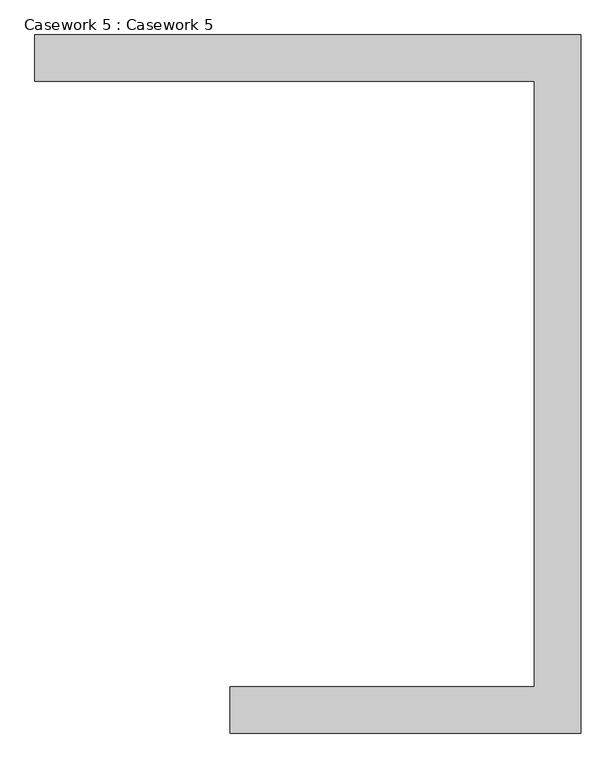
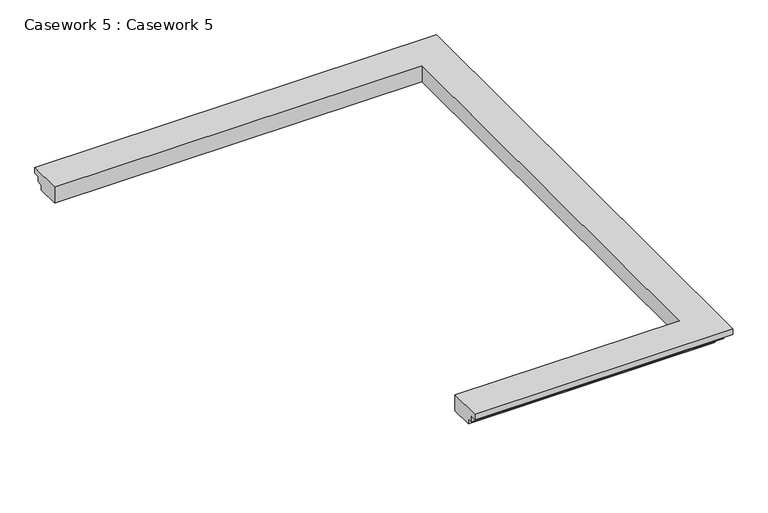
"""IFC4 building model written with IfcOpenShell, lengths in millimetres: furniture geometry, Casework 5 : Casework 5."""

from ifc_helpers import new_model, si_unit, origin, place, context, project, spatial, faceted_brep, source, transform, mapped, element, save


def casework_5_casework_5_052b1e20(model_context):
    return source(origin(), model_context, "Body", "Brep", [
        faceted_brep([(7590.7046034, -5534.1929163, 4350.0), (7590.7046034, -5934.1929163, 4350.0), (7590.7046034, -5934.1929163, 4450.0), (7590.7046034, -6034.1929163, 4450.0), (7590.7046034, -6034.1929163, 4550.0), (7590.7046034, -6134.1929163, 4550.0), (7590.7046034, -6134.1929163, 4650.0), (7590.7046034, -5534.1929163, 4650.0), (11550.7046034, -5534.1929163, 4350.0), (11550.7046034, 2340.8070837, 4350.0), (5050.7046034, 2340.8070837, 4350.0), (5050.7046034, 2740.8070837, 4350.0), (11950.7046034, 2740.8070837, 4350.0), (11950.7046034, -5934.1929163, 4350.0), (11950.7046034, -5934.1929163, 4450.0), (11950.7046034, 2740.8070837, 4450.0), (5050.7046034, 2740.8070837, 4450.0), (5050.7046034, 2840.8070837, 4450.0), (12050.7046034, 2840.8070837, 4450.0), (12050.7046034, -6034.1929163, 4450.0), (12050.7046034, -6034.1929163, 4550.0), (12050.7046034, 2840.8070837, 4550.0), (5050.7046034, 2840.8070837, 4550.0), (5050.7046034, 2940.8070837, 4550.0), (12150.7046034, 2940.8070837, 4550.0), (12150.7046034, -6134.1929163, 4550.0), (12150.7046034, -6134.1929163, 4650.0), (12150.7046034, 2940.8070837, 4650.0), (5050.7046034, 2940.8070837, 4650.0), (5050.7046034, 2340.8070837, 4650.0), (11550.7046034, 2340.8070837, 4650.0), (11550.7046034, -5534.1929163, 4650.0)], [[[0, 1, 2, 3, 4, 5, 6, 7]], [[1, 0, 8, 9, 10, 11, 12, 13]], [[2, 1, 13, 14]], [[3, 2, 14, 15, 16, 17, 18, 19]], [[4, 3, 19, 20]], [[5, 4, 20, 21, 22, 23, 24, 25]], [[6, 5, 25, 26]], [[7, 6, 26, 27, 28, 29, 30, 31]], [[0, 7, 31, 8]], [[14, 13, 12, 15]], [[20, 19, 18, 21]], [[26, 25, 24, 27]], [[8, 31, 30, 9]], [[10, 29, 28, 23, 22, 17, 16, 11]], [[15, 12, 11, 16]], [[21, 18, 17, 22]], [[27, 24, 23, 28]], [[9, 30, 29, 10]]]),
    ])


if __name__ == "__main__":
    model = new_model("IFC4")
    model_context = context("Model", 3, world=origin())
    ifc_project = project(units=[si_unit("LENGTHUNIT", "METRE", prefix="MILLI")], contexts=[model_context])
    site = spatial("IfcSite", under=ifc_project)
    building = spatial("IfcBuilding", under=site)
    placement = place(None, origin())
    casework_5_casework_5_shape = casework_5_casework_5_052b1e20(model_context)
    element("IfcFurniture", 1, ObjectType="Casework 5 : Casework 5", at=placement, inside=building, context=model_context, shape_type="MappedRepresentation", body=[
        mapped(casework_5_casework_5_shape, transform((0.0, 0.0, 0.0), x_axis=(1.0, 0.0, 0.0), y_axis=(0.0, 1.0, 0.0), z_axis=(0.0, 0.0, 1.0))),
    ])
    save(model, "model.ifc")
